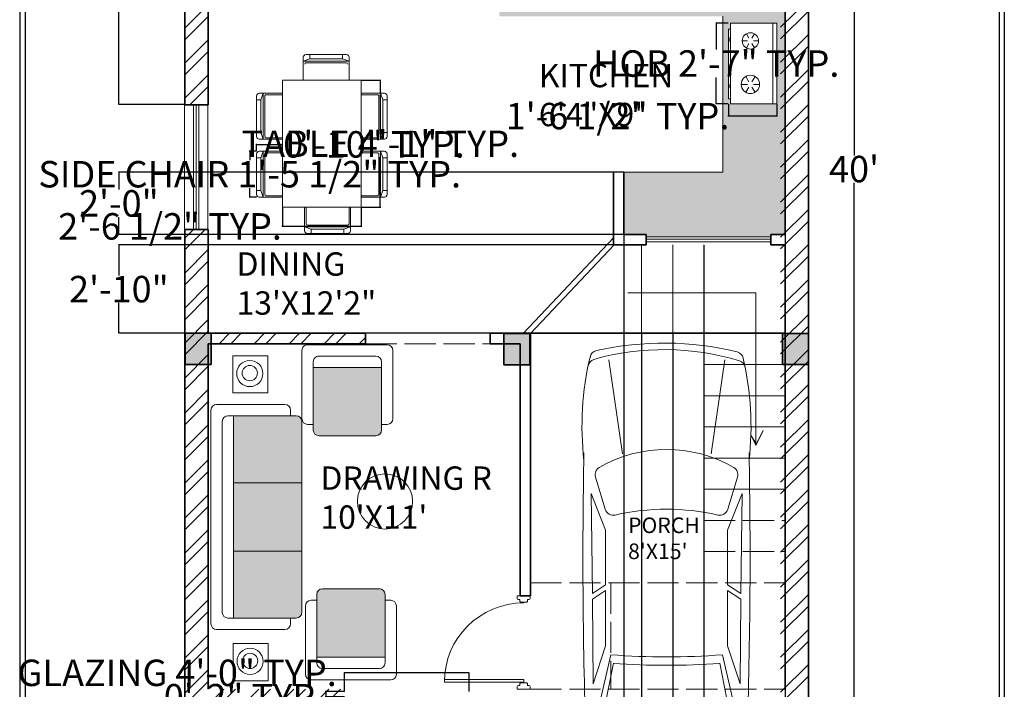
# Model space of a CAD drawing. Units: inches. Extents: x 1812 to 2791, y 2306 to 2959.
# Tile 2 of 8: x 1827 to 2206, y 2458 to 2715. Entities that reach past the tile are written whole.
import ezdxf

# ---------------------------------------------------------------- set-up
doc = ezdxf.new("R2010")
doc.units = ezdxf.units.IN
doc.linetypes.add('ACAD_ISO02W100', pattern=[15, 12, -3])
doc.layers.get('Defpoints').update_dxf_attribs({"lineweight": 50})
for name, color, linetype, lineweight in [('00 FURNITURE', 15, 'Continuous', 15), ('A-ANNO-DIMS', 2, 'Continuous', 18), ('A-ANNO-SYMB', 7, 'Continuous', 18), ('A-ANNO-TTLB', 7, 'Continuous', 25), ('A-AREA-IDEN', 7, 'Continuous', 18), ('A-COLS', 7, 'Continuous', 35), ('A-EQPM', 8, 'Continuous', 18), ('A-FLOR-CASE', 8, 'Continuous', 18), ('A-FLOR-STRS-OVHD', 30, 'ACAD_ISO02W100', 13), ('A-FURNITURE', 251, 'Continuous', 5), ('A-SITE-PARK', 8, 'Continuous', 13), ('A-WALL-OVHD', 30, 'ACAD_ISO02W100', 18), ('A-WALL-PATT', 8, 'Continuous', 13), ('DOORS', 4, 'Continuous', 18), ('STAIRCASE', 7, 'Continuous', 18), ('WALL', 7, 'Continuous', 35), ('WINDOWS', 160, 'Continuous', 18)]:
    doc.layers.add(name, color=color, linetype=linetype, lineweight=lineweight)
doc.layers.add('A-FURN-PATT', color=241, linetype='Continuous', lineweight=9, true_color=0xf7abae)
doc.layers.add('FURN3D', color=229, linetype='Continuous', lineweight=5, true_color=0x4a3f41)
doc.styles.get("Standard").update_dxf_attribs({"font": 'arial.ttf'})
doc.dimstyles.get("Standard").update_dxf_attribs({"dimtxt": 10.18, "dimasz": 0.18, "dimexe": 0.18, "dimexo": 0.0625, "dimgap": 0.09, "dimtad": 0, "dimtih": 1, "dimtoh": 1, "dimdec": 0, "dimzin": 0, "dimdsep": 46, "dimlunit": 3, "dimtxsty": 'Standard', "dimcen": 0.09, "dimadec": 0, "dimazin": 0, "dimtfac": 1, "dimtdec": 0, "dimtofl": 0, "dimtmove": 0, "dimatfit": 3, "dimfxl": 1, "dimtolj": 1, "dimtzin": 0, "dimarcsym": 0})

# ---------------------------------------------------------------- blocks, each defined once
blk = doc.blocks.new('CAR')
at = {"layer": 'A-FURNITURE'}
for p, q in [((2677.91, 1665.57), (2683.24, 1629.33)), ((2722.63, 1665.57), (2717.3, 1629.33)), ((2672.85, 1620.44), (2676.61, 1608)), ((2727.48, 1620.44), (2723.73, 1608)), ((2671.15, 1614.07), (2676.73, 1600.01)), ((2671.63, 1575.61), (2671.15, 1614.07)), ((2729.25, 1614.07), (2723.67, 1600.01)), ((2728.77, 1575.61), (2729.25, 1614.07)), ((2676.73, 1600.01), (2676.73, 1578.97)), ((2723.67, 1600.01), (2723.67, 1578.97)), ((2676.73, 1578.97), (2671.63, 1575.61)), ((2676.73, 1576.71), (2671.66, 1573.38)), ((2676.73, 1576.71), (2676.73, 1555.46)), ((2723.67, 1578.97), (2728.77, 1575.61)), ((2723.67, 1576.71), (2723.67, 1555.46)), ((2723.67, 1576.71), (2728.74, 1573.38)), ((2671.9, 1540.91), (2671.66, 1573.38)), ((2728.49, 1540.91), (2728.74, 1573.38)), ((2676.73, 1555.46), (2671.9, 1540.91)), ((2723.67, 1555.46), (2728.49, 1540.91)), ((2678.77, 1552.01), (2672.52, 1524.85)), ((2721.71, 1552.02), (2727.96, 1524.85)), ((2675.22, 1526.01), (2679.74, 1548.74)), ((2725.17, 1526.01), (2720.66, 1548.74)), ((2672.52, 1524.85), (2672.52, 1517.39)), ((2727.96, 1524.85), (2727.96, 1517.39))]:
    blk.add_line(p, q, dxfattribs=at)
for centre, radius, start, end in [((2699.3, 1552.83), 119.14, 76.3976, 102.667), ((2674, 1665.84), 3.34, 104.3452, 166.6607), ((2699.3, 1570.19), 99.28, 73.0347, 105.8141), ((2726.43, 1665.41), 3.34, 13.1156, 74.5941), ((2783.1, 1639.97), 115.47, 166.6607, 186.5655), ((2673.27, 1662.52), 3.34, 107.8179, 168.3942), ((2727.17, 1661.99), 3.34, 11.3249, 70.8826), ((2617.23, 1639.97), 115.47, 353.4345, 13.1156), ((4741.11, 1589.62), 2073.11, 178.89024, 182.01225), ((2700.17, 1579.09), 51.94, 60.0774, 119.9226), ((659.22, 1589.62), 2073.11, 357.98775, 1.10976), ((2675.91, 1621.37), 3.2, 121.1455, 196.7984), ((2724.42, 1621.37), 3.2, 343.2016, 58.8545), ((2679.67, 1608.92), 3.2, 196.7984, 283.6631), ((2700.17, 1519.83), 88.22, 77.0683, 102.9317), ((2720.66, 1608.92), 3.2, 256.3369, 343.2016), ((2700.16, 1829.45), 278.26, 265.5919, 274.4407), ((2700.17, 1827.63), 279.65, 265.7971, 274.2029), ((2700.17, 1663.47), 139.72, 259.6897, 280.3103), ((2674.03, 1521.04), 4.9, 184.3987, 237.5288), ((2726.3, 1521.04), 4.9, 302.4712, 355.6013), ((2672.62, 1516.95), 3.34, 182.1119, 263.4899), ((2700.17, 1791.26), 275.86, 264.0142, 275.9858), ((2727.71, 1516.95), 3.34, 276.5101, 357.8881), ((2700.17, 1790.18), 277.96, 264.2342, 275.7658)]:
    blk.add_arc(centre, radius, start, end, dxfattribs=at)
blk = doc.blocks.new('sofa 6')
for p, q in [((-1044.4, 890), (1044.4, 890)), ((-1100, 166.9), (-1100, 834.3)), ((-933.1, 778.7), (933.1, 778.7)), ((1100, 834.3), (1100, 166.9)), ((-988.8, 55.6), (-988.8, 723.1)), ((988.8, 723.1), (988.8, 55.6)), ((-988.8, 667.5), (988.8, 667.5)), ((-333.8, 667.5), (-333.8, 0)), ((333.7, 667.5), (333.7, 0)), ((-988.8, 111.2), (-1044.4, 111.2)), ((1044.4, 111.2), (988.8, 111.2)), ((933.1, 0), (-933.1, 0))]:
    blk.add_line(p, q)
for centre, start, end in [((-1044.4, 834.3), 90, 180), ((1044.4, 834.3), 0, 90), ((-933.1, 723.1), 90, 180), ((933.1, 723.1), 0, 90), ((-1044.4, 166.9), 180, 270), ((1044.4, 166.9), 270, 0), ((-933.1, 55.6), 180, 270), ((933.1, 55.6), 270, 0)]:
    blk.add_arc(centre, 55.6, start, end)
blk = doc.blocks.new('CHAIR')
at = {"layer": '00 FURNITURE'}
for p, q in [((1776.1, 2600.27), (1776.1, 2626.55)), ((1778.29, 2628.74), (1800.19, 2628.74)), ((1802.38, 2626.55), (1802.38, 2600.27)), ((1773.91, 2624.36), (1776.1, 2624.36)), ((1802.38, 2624.36), (1804.57, 2624.36)), ((1771.72, 2595.89), (1771.72, 2622.17)), ((1806.76, 2622.17), (1806.76, 2595.89)), ((1802.38, 2602.46), (1776.1, 2602.46)), ((1800.19, 2598.08), (1778.29, 2598.08)), ((1804.57, 2593.7), (1773.91, 2593.7))]:
    blk.add_line(p, q, dxfattribs=at)
for centre, start, end in [((1778.29, 2626.55), 90, 180), ((1800.19, 2626.55), 0, 90), ((1773.91, 2622.17), 90, 180), ((1804.57, 2622.17), 0, 90), ((1778.29, 2600.27), 180, 270), ((1800.19, 2600.27), 270, 0), ((1773.91, 2595.89), 180, 270), ((1804.57, 2595.89), 270, 0)]:
    blk.add_arc(centre, 2.19, start, end, dxfattribs=at)
blk = doc.blocks.new('A$C21540130')
at = {"layer": 'FURN3D'}
for p, q in [((1.57, 0), (1.57, 31.11)), ((9.61, 25.31), (8.63, 27.01)), ((10.79, 25.31), (11.77, 27.01)), ((9.02, 24.29, -27.54), (7.06, 24.29, -27.54)), ((9.61, 23.27), (8.63, 21.57)), ((10.79, 23.27), (11.77, 21.57)), ((11.38, 24.29, -27.54), (13.34, 24.29, -27.54)), ((9.61, 8.56), (8.43, 10.6)), ((10.79, 8.56), (11.97, 10.6)), ((9.02, 7.54), (6.67, 7.54)), ((9.61, 6.52), (8.43, 4.48)), ((10.79, 6.52), (11.97, 4.48)), ((11.38, 7.54), (13.73, 7.54))]:
    blk.add_line(p, q, dxfattribs=at)
for points in [[(0, 0), (0, 31.11), (17.9, 31.11), (17.9, 0)], [(18.68, 1.96), (18.68, 28.83), (17.9, 28.83), (17.9, 1.96)]]:
    blk.add_lwpolyline(points, close=True, dxfattribs=at)
for centre, radius in [((10.2, 24.29), 3.14), ((10.2, 7.54), 3.53)]:
    blk.add_circle(centre, radius, dxfattribs=at)
for points in [[(17.9, 24.03), (18.29, 24.03), (17.9, 25.6), (18.29, 25.6)], [(17.9, 6.05), (18.29, 6.05), (17.9, 7.62), (18.29, 7.62)]]:
    blk.add_solid(points, dxfattribs=at)
blk = doc.blocks.new('DDD')
at = {"layer": '00 FURNITURE'}
for p, q in [((-12579.77, -15859.53), (-12579.77, -15829.05)), ((-12578.77, -15859.53), (-12578.77, -15829.03)), ((-12612.02, -15857.03), (-12612.02, -15862.03)), ((-12611.02, -15857.03), (-12612.02, -15857.03)), ((-12577.02, -15857.03), (-12576.02, -15857.03)), ((-12576.02, -15857.03), (-12576.02, -15862.03)), ((-12610.52, -15858.03), (-12610.52, -15857.53)), ((-12610.52, -15861.53), (-12610.52, -15861.03)), ((-12578.77, -15859.53), (-12579.77, -15859.53)), ((-12577.52, -15858.03), (-12577.52, -15857.53)), ((-12577.52, -15861.53), (-12577.52, -15861.03)), ((-12612.02, -15862.03), (-12611.02, -15862.03)), ((-12576.02, -15862.03), (-12577.02, -15862.03))]:
    blk.add_line(p, q, dxfattribs=at)
for points in [[(-12610.52, -15861.03), (-12610.02, -15861.03, 0.414214), (-12609.52, -15860.53), (-12609.52, -15858.53, 0.414214), (-12610.02, -15858.03), (-12610.52, -15858.03)], [(-12577.52, -15861.03), (-12578.02, -15861.03, -0.414214), (-12578.52, -15860.53), (-12578.52, -15858.53, -0.414214), (-12578.02, -15858.03), (-12577.52, -15858.03)]]:
    blk.add_lwpolyline(points, format="xyb", dxfattribs=at)
for centre, radius, start, end in [((-12578.77, -15859.53), 30.5, 90, 180), ((-12611.02, -15857.53), 0.5, 0, 90), ((-12577.02, -15857.53), 0.5, 90, 180), ((-12611.02, -15861.53), 0.5, 270, 0), ((-12577.02, -15861.53), 0.5, 180, 270)]:
    blk.add_arc(centre, radius, start, end, dxfattribs=at)
blk = doc.blocks.new('*D15')
at = {"layer": 'A-ANNO-DIMS', "color": 0, "lineweight": -2, "transparency": 16777216}
for p, q in [((2130.4, 2898), (2148.13, 2898)), ((2147.95, 2897.82), (2147.95, 2663.08)), ((2147.95, 2417.77), (2147.95, 2652.51)), ((2130.4, 2417.59), (2148.13, 2417.59))]:
    blk.add_line(p, q, dxfattribs=at)
at = {"layer": 'A-ANNO-DIMS', "color": 0, "transparency": 16777216}
for points in [[(2147.92, 2897.82), (2147.98, 2897.82), (2147.95, 2898)], [(2147.92, 2417.77), (2147.98, 2417.77), (2147.95, 2417.59)]]:
    blk.add_solid(points, dxfattribs=at)
at = {"layer": 'Defpoints', "color": 0, "transparency": 16777216}
for p in [(2130.34, 2898), (2130.34, 2417.59), (2147.95, 2417.59)]:
    blk.add_point(p, dxfattribs=at)
at = {"layer": 'A-ANNO-DIMS', "color": 0, "transparency": 16777216, "insert": (2147.95, 2657.8), "char_height": 10.18, "attachment_point": 5}
blk.add_mtext("\\A1;40'", dxfattribs=at)
blk = doc.blocks.new('COL')
at = {"transparency": 33554687}
h = blk.add_hatch(color=256, dxfattribs=at)
h.dxf.hatch_style = 1
h.paths.add_polyline_path([(2424.4, 2829.24), (2424.4, 2839.24), (2412.4, 2839.24), (2412.4, 2829.24)])
for p, q in [((2412.4, 2839.24), (2424.4, 2839.24)), ((2412.4, 2839.24), (2412.4, 2829.24)), ((2424.4, 2839.24), (2424.4, 2829.24)), ((2412.4, 2829.24), (2424.4, 2829.24))]:
    blk.add_line(p, q)
blk = doc.blocks.new('CHAIR-DINING')
for p, q in [((0, 16.64), (0, 1.02)), ((9.93, 17.65), (1.02, 17.65)), ((1.61, 15.13), (2.57, 17.65)), ((2.57, 17.65), (2.57, 0)), ((3.13, 16.53), (3.13, 1.12)), ((9.93, 17.09), (3.69, 17.09)), ((1.61, 15.13), (1.61, 2.55)), ((1.61, 2.55), (2.57, 0)), ((3.69, 0.56), (9.93, 0.56)), ((1.02, 0), (9.93, 0))]:
    blk.add_line(p, q)
blk.add_lwpolyline([(0, 15.13), (0, 2.55), (1.61, 2.55), (1.61, 15.13)], close=True)
for centre, radius, start, end in [((1.02, 16.64), 1.02, 89.9999, 179.9999), ((3.69, 16.53), 0.56, 89.9999, 179.9999), ((1.02, 1.02), 1.02, 179.9999, 269.9999), ((3.69, 1.12), 0.56, 179.9999, 269.9999)]:
    blk.add_arc(centre, radius, start, end)
blk = doc.blocks.new('CHAIR-DINING-END')
for p, q in [((0, 8.91), (0, 0)), ((2.55, 8.31), (0, 7.36)), ((16.64, 9.93), (1.02, 9.93)), ((15.13, 8.31), (2.55, 8.31)), ((15.13, 8.31), (17.66, 7.36)), ((17.66, 0), (17.66, 8.91)), ((17.66, 7.36), (0, 7.36)), ((16.53, 6.79), (1.12, 6.79))]:
    blk.add_line(p, q)
blk.add_lwpolyline([(15.13, 9.93), (2.55, 9.93), (2.55, 8.31), (15.13, 8.31)], close=True)
for centre, radius, start, end in [((1.02, 8.91), 1.02, 89.9999, 179.9999), ((16.64, 8.91), 1.02, 359.9999, 89.9999), ((1.12, 6.23), 0.56, 89.9999, 179.9999), ((16.53, 6.23), 0.56, 359.9999, 89.9999)]:
    blk.add_arc(centre, radius, start, end)
blk = doc.blocks.new('TABLE-DINING-RECT')
for p, q in [((30.35, 48.93), (0, 48.93)), ((0, 48.93), (0, 0)), ((30.35, 48.93), (30.35, 0)), ((30.35, 0), (0, 0))]:
    blk.add_line(p, q)
blk = doc.blocks.new('TABLE-END-SQUARE')
blk.add_lwpolyline([(0, 14.29), (13.46, 14.29), (13.46, 0), (0, 0)], close=True)
for centre, radius in [((6.55, 7.48), 5.04), ((6.52, 7.65), 2.93)]:
    blk.add_circle(centre, radius)
blk = doc.blocks.new('WINDOW-48x9')
for p, q in [((0, 48), (0, 0)), ((3.5, 0), (3.5, 48)), ((4.5, 0), (4.5, 48)), ((5.5, 0), (5.5, 48)), ((9, 0), (9, 48))]:
    blk.add_line(p, q)
blk = doc.blocks.new('STAIR-DIRECTION')
for p, q in [((0, 58.78), (49.24, 58.78)), ((49.24, 58.78), (49.24, 0)), ((49.21, 0.29), (47.33, 4.04)), ((47.33, 4.04), (49.07, 1.3)), ((52.1, 5.77), (49.21, 0.29)), ((49.24, 0), (52.1, 5.77))]:
    blk.add_line(p, q)
blk = doc.blocks.new('SHEET-FRAME-RESIDENCE')
blk.add_lwpolyline([(0, 632.8), (378.76, 632.8), (378.76, 0), (0, 0)], close=True)
blk.add_lwpolyline([(2, 71.32), (2, 630.8), (376.76, 630.8), (376.76, 71.32)])
blk = doc.blocks.new('*D38')
at = {"layer": 'A-ANNO-DIMS', "color": 0, "lineweight": -2, "transparency": 16777216}
for p, q in [((1917.91, 2664.65), (1915.15, 2664.65)), ((1915.33, 2664.47), (1915.33, 2661.18)), ((1915.33, 2647.17), (1915.33, 2650.47)), ((1917.91, 2646.99), (1915.15, 2646.99))]:
    blk.add_line(p, q, dxfattribs=at)
at = {"layer": 'A-ANNO-DIMS', "color": 0, "transparency": 16777216}
for points in [[(1915.3, 2664.47), (1915.36, 2664.47), (1915.33, 2664.65)], [(1915.3, 2647.17), (1915.36, 2647.17), (1915.33, 2646.99)]]:
    blk.add_solid(points, dxfattribs=at)
at = {"layer": 'Defpoints', "color": 0, "transparency": 16777216}
for p in [(1915.33, 2664.65), (1917.98, 2664.65), (1917.98, 2646.99)]:
    blk.add_point(p, dxfattribs=at)
at = {"layer": 'A-ANNO-DIMS', "color": 0, "transparency": 16777216, "insert": (1915.33, 2655.82), "char_height": 10.18, "attachment_point": 5}
blk.add_mtext('\\A1;SIDE CHAIR 1\'-5 1/2" TYP.', dxfattribs=at)
blk = doc.blocks.new('*D39')
at = {"layer": 'A-ANNO-DIMS', "color": 0, "lineweight": -2, "transparency": 16777216}
for p, q in [((1917.98, 2664.71), (1917.98, 2667.48)), ((1918.16, 2667.3), (1927.72, 2667.3)), ((1927.9, 2664.71), (1927.9, 2667.48)), ((1927.9, 2667.3), (1928.08, 2667.3))]:
    blk.add_line(p, q, dxfattribs=at)
at = {"layer": 'A-ANNO-DIMS', "color": 0, "transparency": 16777216}
for points in [[(1918.16, 2667.33), (1918.16, 2667.27), (1917.98, 2667.3)], [(1927.72, 2667.33), (1927.72, 2667.27), (1927.9, 2667.3)]]:
    blk.add_solid(points, dxfattribs=at)
at = {"layer": 'Defpoints', "color": 0, "transparency": 16777216}
for p in [(1917.98, 2664.65), (1927.9, 2667.3), (1927.9, 2664.65)]:
    blk.add_point(p, dxfattribs=at)
at = {"layer": 'A-ANNO-DIMS', "color": 0, "transparency": 16777216, "insert": (1963.15, 2667.3), "char_height": 10.18, "attachment_point": 5}
blk.add_mtext('\\A1;0\'-10" TYP.', dxfattribs=at)
blk = doc.blocks.new('*D62')
at = {"layer": 'A-ANNO-DIMS', "color": 0, "lineweight": -2, "transparency": 16777216}
for p, q in [((2099.52, 2713.96), (2094.73, 2713.96)), ((2094.91, 2713.78), (2094.91, 2703.76)), ((2094.91, 2683.03), (2094.91, 2693.05)), ((2099.52, 2682.85), (2094.73, 2682.85))]:
    blk.add_line(p, q, dxfattribs=at)
at = {"layer": 'A-ANNO-DIMS', "color": 0, "transparency": 16777216}
for points in [[(2094.88, 2713.78), (2094.94, 2713.78), (2094.91, 2713.96)], [(2094.88, 2683.03), (2094.94, 2683.03), (2094.91, 2682.85)]]:
    blk.add_solid(points, dxfattribs=at)
at = {"layer": 'Defpoints', "color": 0, "transparency": 16777216}
for p in [(2094.91, 2713.96), (2099.58, 2713.96), (2099.58, 2682.85)]:
    blk.add_point(p, dxfattribs=at)
at = {"layer": 'A-ANNO-DIMS', "color": 0, "transparency": 16777216, "insert": (2094.91, 2698.41), "char_height": 10.18, "attachment_point": 5}
blk.add_mtext('\\A1;HOB 2\'-7" TYP.', dxfattribs=at)
blk = doc.blocks.new('*D63')
at = {"layer": 'A-ANNO-DIMS', "color": 0, "lineweight": -2, "transparency": 16777216}
for p, q in [((2099.58, 2682.79), (2099.58, 2678.01)), ((2118.26, 2682.79), (2118.26, 2678.01)), ((2099.58, 2678.19), (2099.4, 2678.19)), ((2118.08, 2678.19), (2099.76, 2678.19))]:
    blk.add_line(p, q, dxfattribs=at)
at = {"layer": 'A-ANNO-DIMS', "color": 0, "transparency": 16777216}
for points in [[(2099.76, 2678.22), (2099.76, 2678.16), (2099.58, 2678.19)], [(2118.08, 2678.22), (2118.08, 2678.16), (2118.26, 2678.19)]]:
    blk.add_solid(points, dxfattribs=at)
at = {"layer": 'Defpoints', "color": 0, "transparency": 16777216}
for p in [(2099.58, 2682.85), (2118.26, 2682.85), (2099.58, 2678.19)]:
    blk.add_point(p, dxfattribs=at)
at = {"layer": 'A-ANNO-DIMS', "color": 0, "transparency": 16777216, "insert": (2056.9, 2678.19), "char_height": 10.18, "attachment_point": 5}
blk.add_mtext('\\A1;1\'-6 1/2" TYP.', dxfattribs=at)
blk = doc.blocks.new('*D66')
at = {"layer": 'A-ANNO-DIMS', "color": 0, "lineweight": -2, "transparency": 16777216}
for p, q in [((1958.31, 2692.01), (1965.77, 2692.01)), ((1965.59, 2691.83), (1965.59, 2672.75)), ((1965.59, 2643.26), (1965.59, 2662.34)), ((1958.31, 2643.08), (1965.77, 2643.08))]:
    blk.add_line(p, q, dxfattribs=at)
at = {"layer": 'A-ANNO-DIMS', "color": 0, "transparency": 16777216}
for points in [[(1965.56, 2691.83), (1965.62, 2691.83), (1965.59, 2692.01)], [(1965.56, 2643.26), (1965.62, 2643.26), (1965.59, 2643.08)]]:
    blk.add_solid(points, dxfattribs=at)
at = {"layer": 'Defpoints', "color": 0, "transparency": 16777216}
for p in [(1958.25, 2692.01), (1958.25, 2643.08), (1965.59, 2643.08)]:
    blk.add_point(p, dxfattribs=at)
at = {"layer": 'A-ANNO-DIMS', "color": 0, "transparency": 16777216, "insert": (1965.59, 2667.55), "char_height": 10.18, "attachment_point": 5}
blk.add_mtext('\\A1;TABLE 4\'-1" TYP.', dxfattribs=at)
blk = doc.blocks.new('*D67')
at = {"layer": 'A-ANNO-DIMS', "color": 0, "lineweight": -2, "transparency": 16777216}
for p, q in [((1927.9, 2643.02), (1927.9, 2635.56)), ((1958.25, 2643.02), (1958.25, 2635.56)), ((1927.9, 2635.74), (1927.72, 2635.74)), ((1958.07, 2635.74), (1928.08, 2635.74))]:
    blk.add_line(p, q, dxfattribs=at)
at = {"layer": 'A-ANNO-DIMS', "color": 0, "transparency": 16777216}
for points in [[(1928.08, 2635.77), (1928.08, 2635.71), (1927.9, 2635.74)], [(1958.07, 2635.77), (1958.07, 2635.71), (1958.25, 2635.74)]]:
    blk.add_solid(points, dxfattribs=at)
at = {"layer": 'Defpoints', "color": 0, "transparency": 16777216}
for p in [(1927.9, 2643.08), (1958.25, 2643.08), (1927.9, 2635.74)]:
    blk.add_point(p, dxfattribs=at)
at = {"layer": 'A-ANNO-DIMS', "color": 0, "transparency": 16777216, "insert": (1884.66, 2635.74), "char_height": 10.18, "attachment_point": 5}
blk.add_mtext('\\A1;2\'-6 1/2" TYP.', dxfattribs=at)
blk = doc.blocks.new('*D68')
at = {"layer": 'A-ANNO-DIMS', "color": 0, "lineweight": -2, "transparency": 16777216}
for p, q in [((1951.81, 2463.94), (1951.63, 2463.94)), ((1951.81, 2456.8), (1951.81, 2464.12)), ((1999.63, 2463.94), (1951.99, 2463.94)), ((1999.81, 2456.8), (1999.81, 2464.12))]:
    blk.add_line(p, q, dxfattribs=at)
at = {"layer": 'A-ANNO-DIMS', "color": 0, "transparency": 16777216}
for points in [[(1951.99, 2463.97), (1951.99, 2463.91), (1951.81, 2463.94)], [(1999.63, 2463.97), (1999.63, 2463.91), (1999.81, 2463.94)]]:
    blk.add_solid(points, dxfattribs=at)
at = {"layer": 'Defpoints', "color": 0, "transparency": 16777216}
for p in [(1951.81, 2463.94), (1951.81, 2456.74), (1999.81, 2456.74)]:
    blk.add_point(p, dxfattribs=at)
at = {"layer": 'A-ANNO-DIMS', "color": 0, "transparency": 16777216, "insert": (1887.41, 2463.94), "char_height": 10.18, "attachment_point": 5}
blk.add_mtext('\\A1;GLAZING 4\'-0" TYP.', dxfattribs=at)
blk = doc.blocks.new('*D69')
at = {"layer": 'A-ANNO-DIMS', "color": 0, "lineweight": -2, "transparency": 16777216}
for p, q in [((1951.75, 2456.74), (1944.43, 2456.74)), ((1944.61, 2456.56), (1944.61, 2454.92)), ((1951.75, 2454.74), (1944.43, 2454.74)), ((1944.61, 2454.56), (1944.43, 2454.56)), ((1944.61, 2454.74), (1944.61, 2454.56))]:
    blk.add_line(p, q, dxfattribs=at)
at = {"layer": 'A-ANNO-DIMS', "color": 0, "transparency": 16777216}
for points in [[(1944.58, 2456.56), (1944.64, 2456.56), (1944.61, 2456.74)], [(1944.58, 2454.92), (1944.64, 2454.92), (1944.61, 2454.74)]]:
    blk.add_solid(points, dxfattribs=at)
at = {"layer": 'Defpoints', "color": 0, "transparency": 16777216}
for p in [(1951.81, 2456.74), (1944.61, 2454.74), (1951.81, 2454.74)]:
    blk.add_point(p, dxfattribs=at)
at = {"layer": 'A-ANNO-DIMS', "color": 0, "transparency": 16777216, "insert": (1913.31, 2454.56), "char_height": 10.18, "attachment_point": 5}
blk.add_mtext('\\A1;0\'-2" TYP.', dxfattribs=at)
blk = doc.blocks.new('*D78')
at = {"layer": 'A-ANNO-DIMS', "color": 0, "lineweight": -2, "transparency": 16777216}
for p, q in [((1890.4, 2772.95), (1864.78, 2772.95)), ((1864.96, 2772.77), (1864.96, 2733.15)), ((1864.96, 2682.82), (1864.96, 2722.44)), ((1890.15, 2682.64), (1864.78, 2682.64))]:
    blk.add_line(p, q, dxfattribs=at)
at = {"layer": 'A-ANNO-DIMS', "color": 0, "transparency": 16777216}
for points in [[(1864.93, 2772.77), (1864.99, 2772.77), (1864.96, 2772.95)], [(1864.93, 2682.82), (1864.99, 2682.82), (1864.96, 2682.64)]]:
    blk.add_solid(points, dxfattribs=at)
at = {"layer": 'Defpoints', "color": 0, "transparency": 16777216}
for p in [(1890.46, 2772.95), (1864.96, 2682.64), (1890.21, 2682.64)]:
    blk.add_point(p, dxfattribs=at)
at = {"layer": 'A-ANNO-DIMS', "color": 0, "transparency": 16777216, "insert": (1864.96, 2727.79), "char_height": 10.18, "attachment_point": 5}
blk.add_mtext('\\A1;7\'-6 1/2"', dxfattribs=at)
blk = doc.blocks.new('*D82')
at = {"layer": 'A-ANNO-DIMS', "color": 0, "lineweight": -2, "transparency": 16777216}
for p, q in [((2059.39, 2656.54), (2059.39, 2392.17)), ((2121.39, 2632.54), (2121.39, 2392.17)), ((2059.57, 2392.35), (2076.77, 2392.35)), ((2121.21, 2392.35), (2104.01, 2392.35))]:
    blk.add_line(p, q, dxfattribs=at)
at = {"layer": 'A-ANNO-DIMS', "color": 0, "transparency": 16777216}
for points in [[(2059.57, 2392.38), (2059.57, 2392.32), (2059.39, 2392.35)], [(2121.21, 2392.38), (2121.21, 2392.32), (2121.39, 2392.35)]]:
    blk.add_solid(points, dxfattribs=at)
at = {"layer": 'Defpoints', "color": 0, "transparency": 16777216}
for p in [(2059.39, 2656.6), (2121.39, 2632.6), (2121.39, 2392.35)]:
    blk.add_point(p, dxfattribs=at)
at = {"layer": 'A-ANNO-DIMS', "color": 0, "transparency": 16777216, "insert": (2090.39, 2392.35), "char_height": 10.18, "attachment_point": 5}
blk.add_mtext('\\A1;5\'-2"', dxfattribs=at)
blk = doc.blocks.new('*D84')
at = {"layer": 'A-ANNO-DIMS', "color": 0, "lineweight": -2, "transparency": 16777216}
for p, q in [((2059.32, 2656.6), (1864.78, 2656.6)), ((1864.96, 2656.42), (1864.96, 2649.89)), ((1864.96, 2632.78), (1864.96, 2639.32)), ((2059.32, 2632.6), (1864.78, 2632.6))]:
    blk.add_line(p, q, dxfattribs=at)
at = {"layer": 'A-ANNO-DIMS', "color": 0, "transparency": 16777216}
for points in [[(1864.93, 2656.42), (1864.99, 2656.42), (1864.96, 2656.6)], [(1864.93, 2632.78), (1864.99, 2632.78), (1864.96, 2632.6)]]:
    blk.add_solid(points, dxfattribs=at)
at = {"layer": 'Defpoints', "color": 0, "transparency": 16777216}
for p in [(2059.39, 2656.6), (1864.96, 2632.6), (2059.39, 2632.6)]:
    blk.add_point(p, dxfattribs=at)
at = {"layer": 'A-ANNO-DIMS', "color": 0, "transparency": 16777216, "insert": (1864.96, 2644.6), "char_height": 10.18, "attachment_point": 5}
blk.add_mtext('\\A1;2\'-0"', dxfattribs=at)
blk = doc.blocks.new('*D85')
at = {"layer": 'A-ANNO-DIMS', "color": 0, "lineweight": -2, "transparency": 16777216}
for p, q in [((2055.32, 2628.6), (1864.78, 2628.6)), ((1864.96, 2628.42), (1864.96, 2616.89)), ((1864.96, 2594.78), (1864.96, 2606.32)), ((2023.32, 2594.6), (1864.78, 2594.6))]:
    blk.add_line(p, q, dxfattribs=at)
at = {"layer": 'A-ANNO-DIMS', "color": 0, "transparency": 16777216}
for points in [[(1864.93, 2628.42), (1864.99, 2628.42), (1864.96, 2628.6)], [(1864.93, 2594.78), (1864.99, 2594.78), (1864.96, 2594.6)]]:
    blk.add_solid(points, dxfattribs=at)
at = {"layer": 'Defpoints', "color": 0, "transparency": 16777216}
for p in [(1864.96, 2628.6), (2055.39, 2628.6), (2023.39, 2594.6)]:
    blk.add_point(p, dxfattribs=at)
at = {"layer": 'A-ANNO-DIMS', "color": 0, "transparency": 16777216, "insert": (1864.96, 2611.6), "char_height": 10.18, "attachment_point": 5}
blk.add_mtext('\\A1;2\'-10"', dxfattribs=at)
blk = doc.blocks.new('*D86')
at = {"layer": 'A-ANNO-DIMS', "color": 0, "lineweight": -2, "transparency": 16777216}
for p, q in [((2066.19, 2594.54), (2066.19, 2392.17)), ((2078.19, 2594.54), (2078.19, 2392.17)), ((2066.37, 2392.35), (2078.01, 2392.35)), ((2078.19, 2392.35), (2078.37, 2392.35))]:
    blk.add_line(p, q, dxfattribs=at)
at = {"layer": 'A-ANNO-DIMS', "color": 0, "transparency": 16777216}
for points in [[(2066.37, 2392.38), (2066.37, 2392.32), (2066.19, 2392.35)], [(2078.01, 2392.38), (2078.01, 2392.32), (2078.19, 2392.35)]]:
    blk.add_solid(points, dxfattribs=at)
at = {"layer": 'Defpoints', "color": 0, "transparency": 16777216}
for p in [(2066.19, 2594.6), (2078.19, 2594.6), (2078.19, 2392.35)]:
    blk.add_point(p, dxfattribs=at)
at = {"layer": 'A-ANNO-DIMS', "color": 0, "transparency": 16777216, "insert": (2091.51, 2392.35), "char_height": 10.18, "attachment_point": 5}
blk.add_mtext('\\A1;1\'-0"', dxfattribs=at)
blk = doc.blocks.new('*D87')
at = {"layer": 'A-ANNO-DIMS', "color": 0, "lineweight": -2, "transparency": 16777216}
for p, q in [((2090.19, 2628.54), (2090.19, 2392.17)), ((2121.39, 2628.54), (2121.39, 2392.17)), ((2090.37, 2392.35), (2092.08, 2392.35)), ((2121.21, 2392.35), (2119.49, 2392.35))]:
    blk.add_line(p, q, dxfattribs=at)
at = {"layer": 'A-ANNO-DIMS', "color": 0, "transparency": 16777216}
for points in [[(2090.37, 2392.38), (2090.37, 2392.32), (2090.19, 2392.35)], [(2121.21, 2392.38), (2121.21, 2392.32), (2121.39, 2392.35)]]:
    blk.add_solid(points, dxfattribs=at)
at = {"layer": 'Defpoints', "color": 0, "transparency": 16777216}
for p in [(2090.19, 2628.6), (2121.39, 2628.6), (2121.39, 2392.35)]:
    blk.add_point(p, dxfattribs=at)
at = {"layer": 'A-ANNO-DIMS', "color": 0, "transparency": 16777216, "insert": (2105.79, 2392.35), "char_height": 10.18, "attachment_point": 5}
blk.add_mtext('\\A1;2\'-7"', dxfattribs=at)

msp = doc.modelspace()

# ---------------------------------------------------------------- hatches: boundary and pattern name
at = {"layer": 'A-FURN-PATT', "transparency": 33554534}
h = msp.add_hatch(color=256, dxfattribs=at)
h.dxf.hatch_style = 1
h.paths.add_polyline_path([(2121.39, 2740.6), (2053.61, 2740.6), (2053.61, 2716.6), (2097.39, 2716.6), (2097.39, 2656.6), (2059.39, 2656.6), (2059.39, 2632.6), (2067.87, 2632.6), (2067.87, 2631.77), (2115.87, 2631.77), (2115.87, 2632.6), (2121.39, 2632.6)])
h.paths.add_polyline_path([(2100.36, 2713.96), (2118.26, 2713.96), (2118.26, 2682.85), (2100.36, 2682.85), (2100.36, 2684.81), (2099.58, 2684.81), (2099.58, 2711.69), (2100.36, 2711.69)], flags=16)
h.paths.add_polyline_path([(2111.2, 2707.14, -1), (2104.93, 2707.14, -1)], flags=0)
h.paths.add_polyline_path([(2111.59, 2690.39, -1), (2104.53, 2690.39, -1)], flags=0)
h.paths.add_polyline_path([(2121.35, 2768.56), (2012.67, 2768.56), (2012.67, 2744.6), (2121.35, 2744.6)])
h.paths.add_polyline_path([(2053.61, 2740.6), (2011.39, 2740.6), (2011.39, 2716.6), (2053.61, 2716.6)])
h.paths.add_polyline_path([(1935.43, 2537.08), (1909.15, 2537.08), (1909.15, 2510.8), (1935.43, 2510.8)])
h.paths.add_polyline_path([(1935.43, 2560.67, 0.414214), (1933.24, 2562.86), (1909.15, 2562.86), (1909.15, 2537.08), (1935.43, 2537.08)])
h.paths.add_polyline_path([(1966.09, 2581.45), (1939.81, 2581.45), (1939.81, 2557.36, 0.414214), (1942, 2555.17), (1963.9, 2555.17, 0.414214), (1966.09, 2557.36)])
h.paths.add_polyline_path([(1935.43, 2510.8), (1909.15, 2510.8), (1909.15, 2485.01), (1933.24, 2485.01, 0.414214), (1935.43, 2487.2)])
h.paths.add_polyline_path([(1967.42, 2494.07, 0.414214), (1965.23, 2496.26), (1943.33, 2496.26, 0.414214), (1941.14, 2494.07), (1941.14, 2469.98), (1967.42, 2469.98)])
h.paths.add_polyline_path([(2050.11, 2878.8, 0.308459), (2048.07, 2878.94, 0.065472), (2038.04, 2868.93), (2037.94, 2868.93, 0.386143), (2037.98, 2866.96, 0.011497), (2047.44, 2857.53, 0.265248), (2049.25, 2857.55, 0.066056), (2059.35, 2867.65, 0.308904), (2059.21, 2869.7, 0.059418)])
h.paths.add_polyline_path([(2060.9, 2878.8, 0.308459), (2058.85, 2878.94, 0.027227), (2054.36, 2875.09, -0.033416), (2059.21, 2869.71, -0.379362), (2059.07, 2867.29, -0.036525), (2053.76, 2861.41, 0.027343), (2058.24, 2857.52, 0.262295), (2060.03, 2857.55, 0.066056), (2070.13, 2867.65, 0.308904), (2070, 2869.7, 0.059418)])
h.paths.add_polyline_path([(2092.58, 2824.46), (2079.67, 2811.56), (2091.68, 2811.56, 0.414214), (2092.58, 2812.46)], flags=17)
h.paths.add_polyline_path([(2092.58, 2860.06), (2091.83, 2860.06, 0.052719), (2036.59, 2848.58, 0.295777), (2027.78, 2860.12), (2027.78, 2812.46, 0.414214), (2028.68, 2811.56), (2050.63, 2811.56), (2079.67, 2811.56, 0.253465), (2082.62, 2821.51, 0.253465), (2092.58, 2824.46)])
h.paths.add_polyline_path([(2091.83, 2860.06), (2063.07, 2860.06, -0.016036), (2060.39, 2857.83, -0.429576), (2057.75, 2857.9, -0.015371), (2055.2, 2860.06), (2052.29, 2860.06, -0.016036), (2049.61, 2857.83, -0.334836), (2047.44, 2857.53, -0.003141), (2044.81, 2860.06), (2027.94, 2860.06, -0.292232), (2036.59, 2848.58, -0.052719)], flags=17)
h.paths.add_polyline_path([(2092.59, 2824.47, -0.2538), (2082.62, 2821.51, -0.253465), (2079.67, 2811.56)])
h.paths.add_polyline_path([(2092.58, 2887.16), (2027.78, 2887.16), (2027.78, 2883.51), (2092.58, 2883.51)])
at = {"layer": 'A-WALL-PATT'}
h = msp.add_hatch(dxfattribs=at)
h.set_pattern_fill('ANSI32', color=256)
h.paths.add_polyline_path([(2130.39, 2417.6), (2119.69, 2417.6), (2119.69, 2768.56), (2121.39, 2768.56), (2121.39, 2801.62), (2121.32, 2849.36), (2121.32, 2801.62), (2130.39, 2801.62)])
h.paths.add_polyline_path([(2023.39, 2426.6), (1899.39, 2426.6), (1899.39, 2453.6), (1951.8, 2453.6), (1951.8, 2457.6), (1899.39, 2457.6), (1899.39, 2590.6), (1959.93, 2590.6), (1959.93, 2594.6), (1899.39, 2594.6), (1899.39, 2634.53), (1890.39, 2634.53), (1890.39, 2417.6), (2023.39, 2417.6)])
h.paths.add_polyline_path([(2119.69, 2426.6), (2112.39, 2426.6), (2112.39, 2417.6), (2119.69, 2417.6)])
h.paths.add_polyline_path([(1899.39, 2740.6), (1941.39, 2740.6), (1941.39, 2744.6), (1899.39, 2744.6), (1899.39, 2772.94), (1890.39, 2772.94), (1890.39, 2682.53), (1899.21, 2682.53), (1899.21, 2682.64)])
h.paths.add_polyline_path([(1975.39, 2838.6), (1899.39, 2838.6), (1899.39, 2856.33), (1890.39, 2856.33), (1890.39, 2796.95), (1899.39, 2796.95), (1899.39, 2834.6), (1971.39, 2834.6), (1971.39, 2740.6), (1975.39, 2740.6)])
h.paths.add_polyline_path([(2119.69, 2897.6), (1890.39, 2897.6), (1890.39, 2880.36), (1899.39, 2880.36), (1899.39, 2888.6), (2119.69, 2888.6)])
h.paths.add_polyline_path([(2130.39, 2897.6), (2119.69, 2897.6), (2119.69, 2888.6), (2121.39, 2888.6), (2121.39, 2849.62), (2130.39, 2849.62)])

# ---------------------------------------------------------------- linework, layer by layer
at = {"layer": '00 FURNITURE'}
msp.add_circle((1967.4, 2529.9), 10.62, dxfattribs=at)
at = {"layer": 'A-FLOR-CASE'}
for p in [(2097.39, 2716.6), (2055.39, 2656.6)]:
    msp.add_line(p, (2097.39, 2656.6), dxfattribs=at)
at = {"layer": 'A-FLOR-STRS-OVHD'}
for p, q in [((2090.28, 2534.6), (2090.28, 2457.6)), ((2090.19, 2522.6), (2121.39, 2522.6)), ((2090.19, 2510.6), (2121.39, 2510.6)), ((2023.39, 2498.6), (2121.39, 2498.6)), ((2054.28, 2498.6), (2054.28, 2457.6)), ((2066.28, 2498.6), (2066.28, 2457.6)), ((2078.28, 2498.6), (2078.28, 2457.6))]:
    msp.add_line(p, q, dxfattribs=at)
at = {"layer": 'A-WALL-OVHD'}
for p, q in [((1959.93, 2594.6), (2007.93, 2594.6)), ((1959.93, 2590.6), (2007.93, 2590.6)), ((2023.39, 2457.6), (2121.39, 2457.6))]:
    msp.add_line(p, q, dxfattribs=at)
at = {"layer": 'STAIRCASE'}
for p, q in [((2066.19, 2628.6), (2066.19, 2594.6)), ((2078.19, 2628.6), (2078.19, 2594.6)), ((2090.19, 2628.6), (2090.19, 2534.6)), ((2090.19, 2582.6), (2121.39, 2582.6)), ((2090.19, 2570.6), (2121.39, 2570.6)), ((2090.19, 2558.6), (2121.39, 2558.6)), ((2090.19, 2546.6), (2121.39, 2546.6)), ((2090.19, 2534.6), (2121.39, 2534.6))]:
    msp.add_line(p, q, dxfattribs=at)
at = {"layer": 'WALL'}
for p, q in [((2130.39, 2801.62), (2130.39, 2417.6)), ((1890.39, 2682.53), (1890.39, 2772.94)), ((1899.39, 2682.53), (1899.39, 2740.6)), ((2121.39, 2740.6), (2121.39, 2632.6)), ((1890.39, 2682.53), (1899.39, 2682.53)), ((2055.39, 2628.6), (2055.39, 2656.6)), ((2059.39, 2632.6), (2059.39, 2656.6)), ((1890.39, 2417.6), (1890.39, 2634.53)), ((1890.39, 2634.53), (1899.39, 2634.53)), ((1899.39, 2594.6), (1899.39, 2634.53)), ((2020.69, 2594.6), (2055.39, 2631.28)), ((2059.39, 2632.6), (2067.87, 2632.6)), ((2067.87, 2628.6), (2067.87, 2632.6)), ((2115.87, 2628.6), (2115.87, 2632.6)), ((2115.87, 2632.6), (2121.39, 2632.6)), ((2023.39, 2594.54), (2055.6, 2628.6)), ((2055.39, 2628.6), (2067.87, 2628.6)), ((2115.87, 2628.6), (2121.39, 2628.6)), ((2121.39, 2628.6), (2121.39, 2457.6)), ((1899.39, 2594.6), (1959.93, 2594.6)), ((1959.93, 2590.6), (1959.93, 2594.6)), ((2007.93, 2590.6), (2007.93, 2594.6)), ((2007.93, 2594.6), (2121.39, 2594.6)), ((2023.39, 2493.6), (2023.39, 2594.6)), ((1899.39, 2590.6), (1959.93, 2590.6)), ((1899.39, 2457.6), (1899.39, 2590.6)), ((2007.93, 2590.6), (2019.39, 2590.6)), ((2019.39, 2493.6), (2019.39, 2590.6)), ((2023.39, 2493.6), (2019.39, 2493.6))]:
    msp.add_line(p, q, dxfattribs=at)
at = {"layer": 'WINDOWS'}
for p, q in [((2115.74, 2631.77), (2067.74, 2631.77)), ((2115.74, 2630.77), (2067.74, 2630.77)), ((2115.74, 2629.77), (2067.74, 2629.77))]:
    msp.add_line(p, q, dxfattribs=at)

# ---------------------------------------------------------------- block references
at = {"layer": '00 FURNITURE'}
for name, p in [('CHAIR-DINING-END', (1935.93, 2691.9)), ('CHAIR-DINING', (1917.98, 2669.32)), ('CHAIR-DINING', (1917.98, 2646.99)), ('TABLE-END-SQUARE', (1908.82, 2571.63)), ('CHAIR', (165.04, -132.48)), ('TABLE-END-SQUARE', (1908.94, 2460.88))]:
    msp.add_blockref(name, p, dxfattribs=at)
for name, p, rotation in [('TABLE-DINING-RECT', (1958.25, 2692.01), 179.9999947369858), ('CHAIR', (3742.19, 5183.91), 180)]:
    msp.add_blockref(name, p, dxfattribs=dict(at, rotation=rotation))
at = {"layer": '00 FURNITURE', "extrusion": (0, 0, -1), "zscale": -1}
for p in [(-1968.18, 2669.32), (-1968.18, 2646.99)]:
    msp.add_blockref('CHAIR-DINING', p, dxfattribs=at)
at = {"layer": '00 FURNITURE', "extrusion": (0, 0, -1), "zscale": -1, "rotation": 90.0000000002938}
msp.add_blockref('CHAIR-DINING', (-1936.47, 2633.05), dxfattribs=at)
at = {"layer": '00 FURNITURE', "xscale": -0.0393700787401575, "yscale": 0.0393700787401575, "zscale": 0.0393700787401575, "rotation": 90}
msp.add_blockref('sofa 6', (1935.43, 2523.94), dxfattribs=at)
at = {"layer": 'A-ANNO-SYMB'}
msp.add_blockref('STAIR-DIRECTION', (2060.88, 2551.39), dxfattribs=at)
at = {"layer": 'A-ANNO-TTLB'}
msp.add_blockref('SHEET-FRAME-RESIDENCE', (1827.03, 2306.12), dxfattribs=at)
at = {"layer": 'A-COLS', "rotation": 270}
for p in [(-938.81, 5006.99), (-816.13, 5006.91), (-708.85, 5006.98)]:
    msp.add_blockref('COL', p, dxfattribs=at)
at = {"layer": 'A-EQPM', "xscale": -1}
msp.add_blockref('A$C21540130', (2118.26, 2682.85), dxfattribs=at)
at = {"layer": 'A-SITE-PARK'}
msp.add_blockref('CAR', (-624.41, 918.86), dxfattribs=at)
at = {"layer": 'DOORS', "xscale": -1, "rotation": 90}
msp.add_blockref('DDD', (-13838.75, -10118.39), dxfattribs=at)
at = {"layer": 'WINDOWS'}
msp.add_blockref('WINDOW-48x9', (1890.21, 2634.64), dxfattribs=at)

# ---------------------------------------------------------------- texts
at = {"layer": 'A-AREA-IDEN', "attachment_point": 1}
for s, width, insert, char_height in [('KITCHEN\\P6\'4"X9\'', 96.4869, (2026.63, 2698.29), 9), ('DINING\\P13\'X12\'2"', 96.4869, (1910.27, 2625.76), 9), ("DRAWING R\\P10'X11'", 96.4869, (1942.57, 2543.37), 9), ("PORCH\\P8'X15'", 184.4395, (2060.97, 2523.71), 6)]:
    msp.add_mtext_dynamic_manual_height_columns(s, width=width, gutter_width=12.5, heights=[0], dxfattribs=dict(at, insert=insert, char_height=char_height))

# ---------------------------------------------------------------- dimensions: what is measured, and where the dimension line sits
at = {"layer": 'A-ANNO-DIMS'}
dim = msp.add_linear_dim(base=(2147.95, 2417.59), p1=(2130.34, 2898), p2=(2130.34, 2417.59), angle=90, dimstyle='Standard', override={"dimclrd": 0, "dimclre": 0, "dimclrt": 0}, dxfattribs=at)
dim.commit()
dim.dimension.update_dxf_attribs({"geometry": '*D15', "text_midpoint": (2147.95, 2657.8), "dimtype": 160})
for base, p1, p2, picture, middle in [((1864.96, 2682.64), (1890.46, 2772.95), (1890.21, 2682.64), '*D78', (1864.96, 2727.79)), ((1864.96, 2632.6), (2059.39, 2656.6), (2059.39, 2632.6), '*D84', (1864.96, 2644.6)), ((1864.96, 2628.6), (2023.39, 2594.6), (2055.39, 2628.6), '*D85', (1864.96, 2611.6))]:
    dim = msp.add_linear_dim(base=base, p1=p1, p2=p2, angle=90, dimstyle='Standard', override={"dimdec": 1, "dimlfac": 1, "dimrnd": 0, "dimzin": 1, "dimdsep": 46, "dimlunit": 4, "dimfrac": 2}, dxfattribs=at)
    dim.commit()
    dim.dimension.update_dxf_attribs({"geometry": picture, "text_midpoint": middle})
for base, p1, p2, angle, text, picture, middle in [((2094.91, 2713.96), (2099.58, 2682.85), (2099.58, 2713.96), 90, 'HOB <> TYP.', '*D62', (2094.91, 2698.41)), ((2099.58, 2678.19), (2118.26, 2682.85), (2099.58, 2682.85), 180, '<> TYP.', '*D63', (2056.9, 2678.19)), ((1915.33, 2664.65), (1917.98, 2646.99), (1917.98, 2664.65), 90, 'SIDE CHAIR <> TYP.', '*D38', (1915.33, 2655.82)), ((1965.59, 2643.08), (1958.25, 2692.01), (1958.25, 2643.08), 270, 'TABLE <> TYP.', '*D66', (1965.59, 2667.55)), ((1927.9018, 2635.7431), (1958.2504, 2643.0822), (1927.9018, 2643.0822), 180, '<> TYP.', '*D67', (1884.6584, 2635.7431)), ((1951.81, 2463.94), (1999.81, 2456.74), (1951.81, 2456.74), 180, 'GLAZING <> TYP.', '*D68', (1887.41, 2463.94)), ((1944.61, 2454.74), (1951.81, 2456.74), (1951.81, 2454.74), 270, '<> TYP.', '*D69', (1913.31, 2454.56))]:
    dim = msp.add_linear_dim(base=base, p1=p1, p2=p2, angle=angle, text=text, dimstyle='Standard', override={"dimdec": 1, "dimlfac": 1, "dimrnd": 0, "dimzin": 1, "dimdsep": 46, "dimlunit": 4, "dimfrac": 2}, dxfattribs=at)
    dim.commit()
    dim.dimension.update_dxf_attribs({"geometry": picture, "text_midpoint": middle})
dim = msp.add_linear_dim(base=(1927.9, 2667.3), p1=(1917.98, 2664.65), p2=(1927.9, 2664.65), text='<> TYP.', dimstyle='Standard', override={"dimdec": 1, "dimlfac": 1, "dimrnd": 0, "dimzin": 1, "dimdsep": 46, "dimlunit": 4, "dimfrac": 2}, dxfattribs=at)
dim.commit()
dim.dimension.update_dxf_attribs({"geometry": '*D39', "text_midpoint": (1963.15, 2667.3)})
for base, p1, p2, picture, middle in [((2121.39, 2392.35), (2059.39, 2656.6), (2121.39, 2632.6), '*D82', (2090.39, 2392.35)), ((2121.39, 2392.35), (2090.19, 2628.6), (2121.39, 2628.6), '*D87', (2105.79, 2392.35)), ((2078.19, 2392.35), (2066.19, 2594.6), (2078.19, 2594.6), '*D86', (2091.51, 2392.35))]:
    dim = msp.add_linear_dim(base=base, p1=p1, p2=p2, dimstyle='Standard', override={"dimdec": 1, "dimlfac": 1, "dimrnd": 0, "dimzin": 1, "dimdsep": 46, "dimlunit": 4, "dimfrac": 2}, dxfattribs=at)
    dim.commit()
    dim.dimension.update_dxf_attribs({"geometry": picture, "text_midpoint": middle})

doc.saveas('drawing.dxf')
